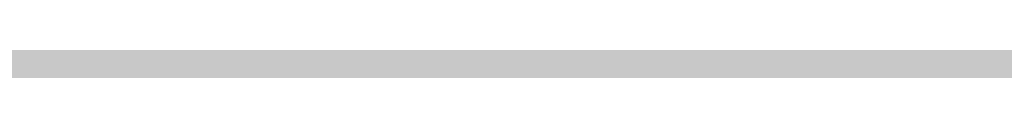
# Model space of a CAD drawing. Units: millimetres. Extents: x -22994 to 29398, y -19990 to 20176.
# Tile 90 of 135: x 229.428 to 230.597, y 83.535 to 83.549. Entities that reach past the tile are written whole.
import ezdxf
from ezdxf import colors
from ezdxf.entities.mleader import LeaderData, LeaderLine
from ezdxf.math import Vec2, Vec3

# ---------------------------------------------------------------- set-up
doc = ezdxf.new("R2010")
doc.units = ezdxf.units.MM
doc.header["$MEASUREMENT"] = 0
doc.layers.add('M-ANNO-TEXT', color=7, linetype='Continuous', lineweight=25)
doc.layers.add('M-DIMS', color=2, linetype='Continuous', lineweight=18)
doc.styles.get("Standard").update_dxf_attribs({"font": 'arial.ttf'})
doc.dimstyles.get("Standard").update_dxf_attribs({"dimtxt": 0.18, "dimasz": 10000, "dimexe": 0.18, "dimexo": 0.0625, "dimgap": 0.09, "dimtad": 0, "dimtih": 1, "dimtoh": 1, "dimdec": 0, "dimzin": 0, "dimdsep": 46, "dimtxsty": 'Standard', "dimcen": 0.09, "dimadec": 0, "dimazin": 0, "dimtfac": 1, "dimtdec": 0, "dimtofl": 0, "dimtmove": 0, "dimatfit": 3, "dimfxl": 1, "dimtolj": 1, "dimtzin": 0, "dimlwd": 30, "dimarcsym": 0})

# ---------------------------------------------------------------- blocks, each defined once
blk = doc.blocks.new('*D2')
at = {"layer": 'Defpoints', "color": 0, "transparency": 16777216}
for p in [(6.6773, 10.2713), (290.852, 10.2713), (290.852, -5.0787)]:
    blk.add_point(p, dxfattribs=at)
at = {"layer": 'M-DIMS', "color": 0, "lineweight": -2, "transparency": 16777216}
for p, q in [((6.6773, 10.2088), (6.6773, -5.2587)), ((290.852, 10.2088), (290.852, -5.2587))]:
    blk.add_line(p, q, dxfattribs=at)
at = {"layer": 'M-DIMS', "color": 0, "lineweight": 30, "transparency": 16777216}
for p, q in [((-9993.3227, -5.0787), (-19993.3227, -5.0787)), ((10290.852, -5.0787), (20290.852, -5.0787))]:
    blk.add_line(p, q, dxfattribs=at)
at = {"layer": 'M-DIMS', "color": 0, "transparency": 16777216}
for points in [[(-9993.3227, 1661.5879), (-9993.3227, -1671.7454), (6.6773, -5.0787)], [(10290.852, 1661.5879), (10290.852, -1671.7454), (290.852, -5.0787)]]:
    blk.add_solid(points, dxfattribs=at)
at = {"layer": 'M-DIMS', "color": 0, "transparency": 16777216, "insert": (148.7647, -5.0787), "char_height": 0.18, "attachment_point": 5}
blk.add_mtext('\\A1;284.2', dxfattribs=at)
blk = doc.blocks.new('*D3')
at = {"layer": 'Defpoints', "color": 0, "transparency": 16777216}
for p in [(110.2647, 204.1654), (110.2647, 176.3662), (95.8327, 127.967)]:
    blk.add_point(p, dxfattribs=at)
at = {"layer": 'M-DIMS', "color": 0, "lineweight": -2, "transparency": 16777216}
for p, q in [((95.8327, 128.0295), (95.8327, 204.3454)), ((110.2647, 176.4287), (110.2647, 204.3454))]:
    blk.add_line(p, q, dxfattribs=at)
at = {"layer": 'M-DIMS', "color": 0, "lineweight": 30, "transparency": 16777216}
for p, q in [((-9904.1673, 204.1654), (-19904.1673, 204.1654)), ((10110.2647, 204.1654), (20110.2647, 204.1654))]:
    blk.add_line(p, q, dxfattribs=at)
at = {"layer": 'M-DIMS', "color": 0, "transparency": 16777216}
for points in [[(-9904.1673, 1870.8321), (-9904.1673, -1462.5013), (95.8327, 204.1654)], [(10110.2647, 1870.8321), (10110.2647, -1462.5013), (110.2647, 204.1654)]]:
    blk.add_solid(points, dxfattribs=at)
at = {"layer": 'M-DIMS', "color": 0, "transparency": 16777216, "insert": (103.0487, 204.1654), "char_height": 0.18, "attachment_point": 5}
blk.add_mtext('\\A1;14.432', dxfattribs=at)
blk = doc.blocks.new('*D4')
at = {"layer": 'Defpoints', "color": 0, "transparency": 16777216}
for p in [(116.2647, 204.1654), (110.2647, 176.3662), (116.2647, 176.3662)]:
    blk.add_point(p, dxfattribs=at)
at = {"layer": 'M-DIMS', "color": 0, "lineweight": -2, "transparency": 16777216}
for p, q in [((110.2647, 176.4287), (110.2647, 204.3454)), ((116.2647, 176.4287), (116.2647, 204.3454))]:
    blk.add_line(p, q, dxfattribs=at)
at = {"layer": 'M-DIMS', "color": 0, "lineweight": 30, "transparency": 16777216}
for p, q in [((-9889.7353, 204.1654), (-19889.7353, 204.1654)), ((10116.2647, 204.1654), (20116.2647, 204.1654))]:
    blk.add_line(p, q, dxfattribs=at)
at = {"layer": 'M-DIMS', "color": 0, "transparency": 16777216}
for points in [[(-9889.7353, 1870.8321), (-9889.7353, -1462.5013), (110.2647, 204.1654)], [(10116.2647, 1870.8321), (10116.2647, -1462.5013), (116.2647, 204.1654)]]:
    blk.add_solid(points, dxfattribs=at)
at = {"layer": 'M-DIMS', "color": 0, "transparency": 16777216, "insert": (113.2647, 204.1654), "char_height": 0.18, "attachment_point": 5}
blk.add_mtext('\\A1;6', dxfattribs=at)
blk = doc.blocks.new('*D5')
at = {"layer": 'Defpoints', "color": 0, "transparency": 16777216}
for p in [(181.2647, 204.1654), (116.2647, 176.3662), (181.2647, 176.3662)]:
    blk.add_point(p, dxfattribs=at)
at = {"layer": 'M-DIMS', "color": 0, "lineweight": -2, "transparency": 16777216}
for p, q in [((116.2647, 176.4287), (116.2647, 204.3454)), ((181.2647, 176.4287), (181.2647, 204.3454))]:
    blk.add_line(p, q, dxfattribs=at)
at = {"layer": 'M-DIMS', "color": 0, "lineweight": 30, "transparency": 16777216}
for p, q in [((-9883.7353, 204.1654), (-19883.7353, 204.1654)), ((10181.2647, 204.1654), (20181.2647, 204.1654))]:
    blk.add_line(p, q, dxfattribs=at)
at = {"layer": 'M-DIMS', "color": 0, "transparency": 16777216}
for points in [[(-9883.7353, 1870.8321), (-9883.7353, -1462.5013), (116.2647, 204.1654)], [(10181.2647, 1870.8321), (10181.2647, -1462.5013), (181.2647, 204.1654)]]:
    blk.add_solid(points, dxfattribs=at)
at = {"layer": 'M-DIMS', "color": 0, "transparency": 16777216, "insert": (148.7647, 204.1654), "char_height": 0.18, "attachment_point": 5}
blk.add_mtext('\\A1;65', dxfattribs=at)
blk = doc.blocks.new('*D6')
at = {"layer": 'Defpoints', "color": 0, "transparency": 16777216}
for p in [(187.2647, 204.1654), (181.2647, 176.3662), (187.2647, 176.3662)]:
    blk.add_point(p, dxfattribs=at)
at = {"layer": 'M-DIMS', "color": 0, "lineweight": -2, "transparency": 16777216}
for p, q in [((181.2647, 176.4287), (181.2647, 204.3454)), ((187.2647, 176.4287), (187.2647, 204.3454))]:
    blk.add_line(p, q, dxfattribs=at)
at = {"layer": 'M-DIMS', "color": 0, "lineweight": 30, "transparency": 16777216}
for p, q in [((-9818.7353, 204.1654), (-19818.7353, 204.1654)), ((10187.2647, 204.1654), (20187.2647, 204.1654))]:
    blk.add_line(p, q, dxfattribs=at)
at = {"layer": 'M-DIMS', "color": 0, "transparency": 16777216}
for points in [[(-9818.7353, 1870.8321), (-9818.7353, -1462.5013), (181.2647, 204.1654)], [(10187.2647, 1870.8321), (10187.2647, -1462.5013), (187.2647, 204.1654)]]:
    blk.add_solid(points, dxfattribs=at)
at = {"layer": 'M-DIMS', "color": 0, "transparency": 16777216, "insert": (184.2647, 204.1654), "char_height": 0.18, "attachment_point": 5}
blk.add_mtext('\\A1;6', dxfattribs=at)
blk = doc.blocks.new('*D7')
at = {"layer": 'Defpoints', "color": 0, "transparency": 16777216}
for p in [(201.6967, 204.1654), (187.2647, 176.3662), (201.6967, 127.967)]:
    blk.add_point(p, dxfattribs=at)
at = {"layer": 'M-DIMS', "color": 0, "lineweight": -2, "transparency": 16777216}
for p, q in [((187.2647, 176.4287), (187.2647, 204.3454)), ((201.6967, 128.0295), (201.6967, 204.3454))]:
    blk.add_line(p, q, dxfattribs=at)
at = {"layer": 'M-DIMS', "color": 0, "lineweight": 30, "transparency": 16777216}
for p, q in [((-9812.7353, 204.1654), (-19812.7353, 204.1654)), ((10201.6967, 204.1654), (20201.6967, 204.1654))]:
    blk.add_line(p, q, dxfattribs=at)
at = {"layer": 'M-DIMS', "color": 0, "transparency": 16777216}
for points in [[(-9812.7353, 1870.8321), (-9812.7353, -1462.5013), (187.2647, 204.1654)], [(10201.6967, 1870.8321), (10201.6967, -1462.5013), (201.6967, 204.1654)]]:
    blk.add_solid(points, dxfattribs=at)
at = {"layer": 'M-DIMS', "color": 0, "transparency": 16777216, "insert": (194.4807, 204.1654), "char_height": 0.18, "attachment_point": 5}
blk.add_mtext('\\A1;14.432', dxfattribs=at)
blk = doc.blocks.new('*D8')
at = {"layer": 'Defpoints', "color": 0, "transparency": 16777216}
for p in [(227.6485, 204.1654), (227.6485, 146.7296), (201.6967, 127.967)]:
    blk.add_point(p, dxfattribs=at)
at = {"layer": 'M-DIMS', "color": 0, "lineweight": -2, "transparency": 16777216}
for p, q in [((201.6967, 128.0295), (201.6967, 204.3454)), ((227.6485, 146.7921), (227.6485, 204.3454))]:
    blk.add_line(p, q, dxfattribs=at)
at = {"layer": 'M-DIMS', "color": 0, "lineweight": 30, "transparency": 16777216}
for p, q in [((-9798.3033, 204.1654), (-19798.3033, 204.1654)), ((10227.6485, 204.1654), (20227.6485, 204.1654))]:
    blk.add_line(p, q, dxfattribs=at)
at = {"layer": 'M-DIMS', "color": 0, "transparency": 16777216}
for points in [[(-9798.3033, 1870.8321), (-9798.3033, -1462.5013), (201.6967, 204.1654)], [(10227.6485, 1870.8321), (10227.6485, -1462.5013), (227.6485, 204.1654)]]:
    blk.add_solid(points, dxfattribs=at)
at = {"layer": 'M-DIMS', "color": 0, "transparency": 16777216, "insert": (214.6726, 204.1654), "char_height": 0.18, "attachment_point": 5}
blk.add_mtext('\\A1;25.95', dxfattribs=at)
blk = doc.blocks.new('*D9')
at = {"layer": 'Defpoints', "color": 0, "transparency": 16777216}
for p in [(187.2647, 176.3662), (306.202, 176.3662), (290.852, 10.2713)]:
    blk.add_point(p, dxfattribs=at)
at = {"layer": 'M-DIMS', "color": 0, "lineweight": 30, "transparency": 16777216}
for p, q in [((306.202, 10176.3662), (306.202, 20176.3662)), ((306.202, -9989.7287), (306.202, -19989.7287))]:
    blk.add_line(p, q, dxfattribs=at)
at = {"layer": 'M-DIMS', "color": 0, "lineweight": -2, "transparency": 16777216}
for p, q in [((187.3272, 176.3662), (306.382, 176.3662)), ((290.9145, 10.2713), (306.382, 10.2713))]:
    blk.add_line(p, q, dxfattribs=at)
at = {"layer": 'M-DIMS', "color": 0, "transparency": 16777216}
for points in [[(-1360.4646, 10176.3662), (1972.8687, 10176.3662), (306.202, 176.3662)], [(-1360.4646, -9989.7287), (1972.8687, -9989.7287), (306.202, 10.2713)]]:
    blk.add_solid(points, dxfattribs=at)
at = {"layer": 'M-DIMS', "color": 0, "transparency": 16777216, "insert": (306.202, 93.3187), "char_height": 0.18, "attachment_point": 5}
blk.add_mtext('\\A1;166.1', dxfattribs=at)
blk = doc.blocks.new('*D10')
at = {"layer": 'Defpoints', "color": 0, "transparency": 16777216}
for p in [(125.6498, 136.0713), (133.3459, 136.0713), (133.3459, -5.0787)]:
    blk.add_point(p, dxfattribs=at)
at = {"layer": 'M-DIMS', "color": 0, "lineweight": -2, "transparency": 16777216}
for p, q in [((125.6498, 136.0088), (125.6498, -5.2587)), ((133.3459, 136.0088), (133.3459, -5.2587))]:
    blk.add_line(p, q, dxfattribs=at)
at = {"layer": 'M-DIMS', "color": 0, "lineweight": 30, "transparency": 16777216}
for p, q in [((-9874.3502, -5.0787), (-19874.3502, -5.0787)), ((10133.3459, -5.0787), (20133.3459, -5.0787))]:
    blk.add_line(p, q, dxfattribs=at)
at = {"layer": 'M-DIMS', "color": 0, "transparency": 16777216}
for points in [[(-9874.3502, 1661.5879), (-9874.3502, -1671.7454), (125.6498, -5.0787)], [(10133.3459, 1661.5879), (10133.3459, -1671.7454), (133.3459, -5.0787)]]:
    blk.add_solid(points, dxfattribs=at)
at = {"layer": 'M-DIMS', "color": 0, "transparency": 16777216, "insert": (129.4978, -5.0787), "char_height": 0.18, "attachment_point": 5}
blk.add_mtext('\\A1;7.696', dxfattribs=at)
blk = doc.blocks.new('*D11')
at = {"layer": 'Defpoints', "color": 0, "transparency": 16777216}
for p in [(133.3459, 136.0713), (135.6498, 136.0713), (135.6498, -5.0787)]:
    blk.add_point(p, dxfattribs=at)
at = {"layer": 'M-DIMS', "color": 0, "lineweight": -2, "transparency": 16777216}
for p, q in [((133.3459, 136.0088), (133.3459, -5.2587)), ((135.6498, 136.0088), (135.6498, -5.2587))]:
    blk.add_line(p, q, dxfattribs=at)
at = {"layer": 'M-DIMS', "color": 0, "lineweight": 30, "transparency": 16777216}
for p, q in [((-9866.6541, -5.0787), (-19866.6541, -5.0787)), ((10135.6498, -5.0787), (20135.6498, -5.0787))]:
    blk.add_line(p, q, dxfattribs=at)
at = {"layer": 'M-DIMS', "color": 0, "transparency": 16777216}
for points in [[(-9866.6541, 1661.5879), (-9866.6541, -1671.7454), (133.3459, -5.0787)], [(10135.6498, 1661.5879), (10135.6498, -1671.7454), (135.6498, -5.0787)]]:
    blk.add_solid(points, dxfattribs=at)
at = {"layer": 'M-DIMS', "color": 0, "transparency": 16777216, "insert": (134.4978, -5.0787), "char_height": 0.18, "attachment_point": 5}
blk.add_mtext('\\A1;2.304', dxfattribs=at)
blk = doc.blocks.new('*D12')
at = {"layer": 'Defpoints', "color": 0, "transparency": 16777216}
for p in [(135.6498, 136.0713), (145.6498, 136.0713), (145.6498, -5.0787)]:
    blk.add_point(p, dxfattribs=at)
at = {"layer": 'M-DIMS', "color": 0, "lineweight": -2, "transparency": 16777216}
for p, q in [((135.6498, 136.0088), (135.6498, -5.2587)), ((145.6498, 136.0088), (145.6498, -5.2587))]:
    blk.add_line(p, q, dxfattribs=at)
at = {"layer": 'M-DIMS', "color": 0, "lineweight": 30, "transparency": 16777216}
for p, q in [((-9864.3502, -5.0787), (-19864.3502, -5.0787)), ((10145.6498, -5.0787), (20145.6498, -5.0787))]:
    blk.add_line(p, q, dxfattribs=at)
at = {"layer": 'M-DIMS', "color": 0, "transparency": 16777216}
for points in [[(-9864.3502, 1661.5879), (-9864.3502, -1671.7454), (135.6498, -5.0787)], [(10145.6498, 1661.5879), (10145.6498, -1671.7454), (145.6498, -5.0787)]]:
    blk.add_solid(points, dxfattribs=at)
at = {"layer": 'M-DIMS', "color": 0, "transparency": 16777216, "insert": (140.6498, -5.0787), "char_height": 0.18, "attachment_point": 5}
blk.add_mtext('\\A1;10', dxfattribs=at)
blk = doc.blocks.new('*D13')
at = {"layer": 'Defpoints', "color": 0, "transparency": 16777216}
for p in [(145.6498, 136.0713), (155.6498, 136.0713), (155.6498, -5.0787)]:
    blk.add_point(p, dxfattribs=at)
at = {"layer": 'M-DIMS', "color": 0, "lineweight": -2, "transparency": 16777216}
for p, q in [((145.6498, 136.0088), (145.6498, -5.2587)), ((155.6498, 136.0088), (155.6498, -5.2587))]:
    blk.add_line(p, q, dxfattribs=at)
at = {"layer": 'M-DIMS', "color": 0, "lineweight": 30, "transparency": 16777216}
for p, q in [((-9854.3502, -5.0787), (-19854.3502, -5.0787)), ((10155.6498, -5.0787), (20155.6498, -5.0787))]:
    blk.add_line(p, q, dxfattribs=at)
at = {"layer": 'M-DIMS', "color": 0, "transparency": 16777216}
for points in [[(-9854.3502, 1661.5879), (-9854.3502, -1671.7454), (145.6498, -5.0787)], [(10155.6498, 1661.5879), (10155.6498, -1671.7454), (155.6498, -5.0787)]]:
    blk.add_solid(points, dxfattribs=at)
at = {"layer": 'M-DIMS', "color": 0, "transparency": 16777216, "insert": (150.6498, -5.0787), "char_height": 0.18, "attachment_point": 5}
blk.add_mtext('\\A1;10', dxfattribs=at)
blk = doc.blocks.new('*D14')
at = {"layer": 'Defpoints', "color": 0, "transparency": 16777216}
for p in [(155.6498, 136.0713), (165.6498, 136.0713), (165.6498, -5.0787)]:
    blk.add_point(p, dxfattribs=at)
at = {"layer": 'M-DIMS', "color": 0, "lineweight": -2, "transparency": 16777216}
for p, q in [((155.6498, 136.0088), (155.6498, -5.2587)), ((165.6498, 136.0088), (165.6498, -5.2587))]:
    blk.add_line(p, q, dxfattribs=at)
at = {"layer": 'M-DIMS', "color": 0, "lineweight": 30, "transparency": 16777216}
for p, q in [((-9844.3502, -5.0787), (-19844.3502, -5.0787)), ((10165.6498, -5.0787), (20165.6498, -5.0787))]:
    blk.add_line(p, q, dxfattribs=at)
at = {"layer": 'M-DIMS', "color": 0, "transparency": 16777216}
for points in [[(-9844.3502, 1661.5879), (-9844.3502, -1671.7454), (155.6498, -5.0787)], [(10165.6498, 1661.5879), (10165.6498, -1671.7454), (165.6498, -5.0787)]]:
    blk.add_solid(points, dxfattribs=at)
at = {"layer": 'M-DIMS', "color": 0, "transparency": 16777216, "insert": (160.6498, -5.0787), "char_height": 0.18, "attachment_point": 5}
blk.add_mtext('\\A1;10', dxfattribs=at)
blk = doc.blocks.new('*D15')
at = {"layer": 'Defpoints', "color": 0, "transparency": 16777216}
for p in [(173.3459, 154.788), (173.3459, 136.0713), (306.202, 136.0713)]:
    blk.add_point(p, dxfattribs=at)
at = {"layer": 'M-DIMS', "color": 0, "lineweight": 30, "transparency": 16777216}
for p, q in [((306.202, 10154.788), (306.202, 20154.788)), ((306.202, -9863.9287), (306.202, -19863.9287))]:
    blk.add_line(p, q, dxfattribs=at)
at = {"layer": 'M-DIMS', "color": 0, "lineweight": -2, "transparency": 16777216}
for p, q in [((173.4084, 154.788), (306.382, 154.788)), ((173.4084, 136.0713), (306.382, 136.0713))]:
    blk.add_line(p, q, dxfattribs=at)
at = {"layer": 'M-DIMS', "color": 0, "transparency": 16777216}
for points in [[(-1360.4646, 10154.788), (1972.8687, 10154.788), (306.202, 154.788)], [(-1360.4646, -9863.9287), (1972.8687, -9863.9287), (306.202, 136.0713)]]:
    blk.add_solid(points, dxfattribs=at)
at = {"layer": 'M-DIMS', "color": 0, "transparency": 16777216, "insert": (306.202, 145.4297), "char_height": 0.18, "attachment_point": 5}
blk.add_mtext('\\A1;18.717', dxfattribs=at)
blk = doc.blocks.new('*D16')
at = {"layer": 'Defpoints', "color": 0, "transparency": 16777216}
for p in [(120.1702, 204.1654), (110.4658, 48.0349), (120.1702, 48.0349)]:
    blk.add_point(p, dxfattribs=at)
at = {"layer": 'M-DIMS', "color": 0, "lineweight": -2, "transparency": 16777216}
for p, q in [((110.4658, 48.0974), (110.4658, 204.3454)), ((120.1702, 48.0974), (120.1702, 204.3454))]:
    blk.add_line(p, q, dxfattribs=at)
at = {"layer": 'M-DIMS', "color": 0, "lineweight": 30, "transparency": 16777216}
for p, q in [((-9889.5342, 204.1654), (-19889.5342, 204.1654)), ((10120.1702, 204.1654), (20120.1702, 204.1654))]:
    blk.add_line(p, q, dxfattribs=at)
at = {"layer": 'M-DIMS', "color": 0, "transparency": 16777216}
for points in [[(-9889.5342, 1870.8321), (-9889.5342, -1462.5013), (110.4658, 204.1654)], [(10120.1702, 1870.8321), (10120.1702, -1462.5013), (120.1702, 204.1654)]]:
    blk.add_solid(points, dxfattribs=at)
at = {"layer": 'M-DIMS', "color": 0, "transparency": 16777216, "insert": (115.318, 204.1654), "char_height": 0.18, "attachment_point": 5}
blk.add_mtext('\\A1;9.704', dxfattribs=at)
blk = doc.blocks.new('*D17')
at = {"layer": 'Defpoints', "color": 0, "transparency": 16777216}
for p in [(126.1702, 204.1654), (120.1702, 48.0349), (126.1702, 48.0349)]:
    blk.add_point(p, dxfattribs=at)
at = {"layer": 'M-DIMS', "color": 0, "lineweight": -2, "transparency": 16777216}
for p, q in [((120.1702, 48.0974), (120.1702, 204.3454)), ((126.1702, 48.0974), (126.1702, 204.3454))]:
    blk.add_line(p, q, dxfattribs=at)
at = {"layer": 'M-DIMS', "color": 0, "lineweight": 30, "transparency": 16777216}
for p, q in [((-9879.8298, 204.1654), (-19879.8298, 204.1654)), ((10126.1702, 204.1654), (20126.1702, 204.1654))]:
    blk.add_line(p, q, dxfattribs=at)
at = {"layer": 'M-DIMS', "color": 0, "transparency": 16777216}
for points in [[(-9879.8298, 1870.8321), (-9879.8298, -1462.5013), (120.1702, 204.1654)], [(10126.1702, 1870.8321), (10126.1702, -1462.5013), (126.1702, 204.1654)]]:
    blk.add_solid(points, dxfattribs=at)
at = {"layer": 'M-DIMS', "color": 0, "transparency": 16777216, "insert": (123.1702, 204.1654), "char_height": 0.18, "attachment_point": 5}
blk.add_mtext('\\A1;6', dxfattribs=at)
blk = doc.blocks.new('*D18')
at = {"layer": 'Defpoints', "color": 0, "transparency": 16777216}
for p in [(132.1702, 204.1654), (126.1702, 48.0349), (132.1702, 48.0349)]:
    blk.add_point(p, dxfattribs=at)
at = {"layer": 'M-DIMS', "color": 0, "lineweight": -2, "transparency": 16777216}
for p, q in [((126.1702, 48.0974), (126.1702, 204.3454)), ((132.1702, 48.0974), (132.1702, 204.3454))]:
    blk.add_line(p, q, dxfattribs=at)
at = {"layer": 'M-DIMS', "color": 0, "lineweight": 30, "transparency": 16777216}
for p, q in [((-9873.8298, 204.1654), (-19873.8298, 204.1654)), ((10132.1702, 204.1654), (20132.1702, 204.1654))]:
    blk.add_line(p, q, dxfattribs=at)
at = {"layer": 'M-DIMS', "color": 0, "transparency": 16777216}
for points in [[(-9873.8298, 1870.8321), (-9873.8298, -1462.5013), (126.1702, 204.1654)], [(10132.1702, 1870.8321), (10132.1702, -1462.5013), (132.1702, 204.1654)]]:
    blk.add_solid(points, dxfattribs=at)
at = {"layer": 'M-DIMS', "color": 0, "transparency": 16777216, "insert": (129.1702, 204.1654), "char_height": 0.18, "attachment_point": 5}
blk.add_mtext('\\A1;6', dxfattribs=at)
blk = doc.blocks.new('*D19')
at = {"layer": 'Defpoints', "color": 0, "transparency": 16777216}
for p in [(138.1702, 204.1654), (132.1702, 48.0349), (138.1702, 48.0349)]:
    blk.add_point(p, dxfattribs=at)
at = {"layer": 'M-DIMS', "color": 0, "lineweight": -2, "transparency": 16777216}
for p, q in [((132.1702, 48.0974), (132.1702, 204.3454)), ((138.1702, 48.0974), (138.1702, 204.3454))]:
    blk.add_line(p, q, dxfattribs=at)
at = {"layer": 'M-DIMS', "color": 0, "lineweight": 30, "transparency": 16777216}
for p, q in [((-9867.8298, 204.1654), (-19867.8298, 204.1654)), ((10138.1702, 204.1654), (20138.1702, 204.1654))]:
    blk.add_line(p, q, dxfattribs=at)
at = {"layer": 'M-DIMS', "color": 0, "transparency": 16777216}
for points in [[(-9867.8298, 1870.8321), (-9867.8298, -1462.5013), (132.1702, 204.1654)], [(10138.1702, 1870.8321), (10138.1702, -1462.5013), (138.1702, 204.1654)]]:
    blk.add_solid(points, dxfattribs=at)
at = {"layer": 'M-DIMS', "color": 0, "transparency": 16777216, "insert": (135.1702, 204.1654), "char_height": 0.18, "attachment_point": 5}
blk.add_mtext('\\A1;6', dxfattribs=at)
blk = doc.blocks.new('*D20')
at = {"layer": 'Defpoints', "color": 0, "transparency": 16777216}
for p in [(144.1702, 204.1654), (138.1702, 48.0349), (144.1702, 48.0349)]:
    blk.add_point(p, dxfattribs=at)
at = {"layer": 'M-DIMS', "color": 0, "lineweight": -2, "transparency": 16777216}
for p, q in [((138.1702, 48.0974), (138.1702, 204.3454)), ((144.1702, 48.0974), (144.1702, 204.3454))]:
    blk.add_line(p, q, dxfattribs=at)
at = {"layer": 'M-DIMS', "color": 0, "lineweight": 30, "transparency": 16777216}
for p, q in [((-9861.8298, 204.1654), (-19861.8298, 204.1654)), ((10144.1702, 204.1654), (20144.1702, 204.1654))]:
    blk.add_line(p, q, dxfattribs=at)
at = {"layer": 'M-DIMS', "color": 0, "transparency": 16777216}
for points in [[(-9861.8298, 1870.8321), (-9861.8298, -1462.5013), (138.1702, 204.1654)], [(10144.1702, 1870.8321), (10144.1702, -1462.5013), (144.1702, 204.1654)]]:
    blk.add_solid(points, dxfattribs=at)
at = {"layer": 'M-DIMS', "color": 0, "transparency": 16777216, "insert": (141.1702, 204.1654), "char_height": 0.18, "attachment_point": 5}
blk.add_mtext('\\A1;6', dxfattribs=at)
blk = doc.blocks.new('*D21')
at = {"layer": 'Defpoints', "color": 0, "transparency": 16777216}
for p in [(149.1157, 204.1654), (144.1702, 48.0349), (149.1157, 48.0349)]:
    blk.add_point(p, dxfattribs=at)
at = {"layer": 'M-DIMS', "color": 0, "lineweight": -2, "transparency": 16777216}
for p, q in [((144.1702, 48.0974), (144.1702, 204.3454)), ((149.1157, 48.0974), (149.1157, 204.3454))]:
    blk.add_line(p, q, dxfattribs=at)
at = {"layer": 'M-DIMS', "color": 0, "lineweight": 30, "transparency": 16777216}
for p, q in [((-9855.8298, 204.1654), (-19855.8298, 204.1654)), ((10149.1157, 204.1654), (20149.1157, 204.1654))]:
    blk.add_line(p, q, dxfattribs=at)
at = {"layer": 'M-DIMS', "color": 0, "transparency": 16777216}
for points in [[(-9855.8298, 1870.8321), (-9855.8298, -1462.5013), (144.1702, 204.1654)], [(10149.1157, 1870.8321), (10149.1157, -1462.5013), (149.1157, 204.1654)]]:
    blk.add_solid(points, dxfattribs=at)
at = {"layer": 'M-DIMS', "color": 0, "transparency": 16777216, "insert": (146.6429, 204.1654), "char_height": 0.18, "attachment_point": 5}
blk.add_mtext('\\A1;4.945', dxfattribs=at)
blk = doc.blocks.new('*D22')
at = {"layer": 'Defpoints', "color": 0, "transparency": 16777216}
for p in [(149.1157, 30.9895), (155.1157, 30.9895), (155.1157, -5.0787)]:
    blk.add_point(p, dxfattribs=at)
at = {"layer": 'M-DIMS', "color": 0, "lineweight": -2, "transparency": 16777216}
for p, q in [((149.1157, 30.927), (149.1157, -5.2587)), ((155.1157, 30.927), (155.1157, -5.2587))]:
    blk.add_line(p, q, dxfattribs=at)
at = {"layer": 'M-DIMS', "color": 0, "lineweight": 30, "transparency": 16777216}
for p, q in [((-9850.8843, -5.0787), (-19850.8843, -5.0787)), ((10155.1157, -5.0787), (20155.1157, -5.0787))]:
    blk.add_line(p, q, dxfattribs=at)
at = {"layer": 'M-DIMS', "color": 0, "transparency": 16777216}
for points in [[(-9850.8843, 1661.5879), (-9850.8843, -1671.7454), (149.1157, -5.0787)], [(10155.1157, 1661.5879), (10155.1157, -1671.7454), (155.1157, -5.0787)]]:
    blk.add_solid(points, dxfattribs=at)
at = {"layer": 'M-DIMS', "color": 0, "transparency": 16777216, "insert": (152.1157, -5.0787), "char_height": 0.18, "attachment_point": 5}
blk.add_mtext('\\A1;6', dxfattribs=at)
blk = doc.blocks.new('*D23')
at = {"layer": 'Defpoints', "color": 0, "transparency": 16777216}
for p in [(155.1157, 30.9895), (161.1157, 30.9895), (161.1157, -5.0787)]:
    blk.add_point(p, dxfattribs=at)
at = {"layer": 'M-DIMS', "color": 0, "lineweight": -2, "transparency": 16777216}
for p, q in [((155.1157, 30.927), (155.1157, -5.2587)), ((161.1157, 30.927), (161.1157, -5.2587))]:
    blk.add_line(p, q, dxfattribs=at)
at = {"layer": 'M-DIMS', "color": 0, "lineweight": 30, "transparency": 16777216}
for p, q in [((-9844.8843, -5.0787), (-19844.8843, -5.0787)), ((10161.1157, -5.0787), (20161.1157, -5.0787))]:
    blk.add_line(p, q, dxfattribs=at)
at = {"layer": 'M-DIMS', "color": 0, "transparency": 16777216}
for points in [[(-9844.8843, 1661.5879), (-9844.8843, -1671.7454), (155.1157, -5.0787)], [(10161.1157, 1661.5879), (10161.1157, -1671.7454), (161.1157, -5.0787)]]:
    blk.add_solid(points, dxfattribs=at)
at = {"layer": 'M-DIMS', "color": 0, "transparency": 16777216, "insert": (158.1157, -5.0787), "char_height": 0.18, "attachment_point": 5}
blk.add_mtext('\\A1;6', dxfattribs=at)
blk = doc.blocks.new('*D24')
at = {"layer": 'Defpoints', "color": 0, "transparency": 16777216}
for p in [(161.1157, 30.9895), (166.4387, 30.9895), (166.4387, -5.0787)]:
    blk.add_point(p, dxfattribs=at)
at = {"layer": 'M-DIMS', "color": 0, "lineweight": -2, "transparency": 16777216}
for p, q in [((161.1157, 30.927), (161.1157, -5.2587)), ((166.4387, 30.927), (166.4387, -5.2587))]:
    blk.add_line(p, q, dxfattribs=at)
at = {"layer": 'M-DIMS', "color": 0, "lineweight": 30, "transparency": 16777216}
for p, q in [((-9838.8843, -5.0787), (-19838.8843, -5.0787)), ((10166.4387, -5.0787), (20166.4387, -5.0787))]:
    blk.add_line(p, q, dxfattribs=at)
at = {"layer": 'M-DIMS', "color": 0, "transparency": 16777216}
for points in [[(-9838.8843, 1661.5879), (-9838.8843, -1671.7454), (161.1157, -5.0787)], [(10166.4387, 1661.5879), (10166.4387, -1671.7454), (166.4387, -5.0787)]]:
    blk.add_solid(points, dxfattribs=at)
at = {"layer": 'M-DIMS', "color": 0, "transparency": 16777216, "insert": (163.7772, -5.0787), "char_height": 0.18, "attachment_point": 5}
blk.add_mtext('\\A1;5.323', dxfattribs=at)
blk = doc.blocks.new('*D25')
at = {"layer": 'Defpoints', "color": 0, "transparency": 16777216}
for p in [(166.4387, 30.9895), (172.4387, 30.9895), (172.4387, -5.0787)]:
    blk.add_point(p, dxfattribs=at)
at = {"layer": 'M-DIMS', "color": 0, "lineweight": -2, "transparency": 16777216}
for p, q in [((166.4387, 30.927), (166.4387, -5.2587)), ((172.4387, 30.927), (172.4387, -5.2587))]:
    blk.add_line(p, q, dxfattribs=at)
at = {"layer": 'M-DIMS', "color": 0, "lineweight": 30, "transparency": 16777216}
for p, q in [((-9833.5613, -5.0787), (-19833.5613, -5.0787)), ((10172.4387, -5.0787), (20172.4387, -5.0787))]:
    blk.add_line(p, q, dxfattribs=at)
at = {"layer": 'M-DIMS', "color": 0, "transparency": 16777216}
for points in [[(-9833.5613, 1661.5879), (-9833.5613, -1671.7454), (166.4387, -5.0787)], [(10172.4387, 1661.5879), (10172.4387, -1671.7454), (172.4387, -5.0787)]]:
    blk.add_solid(points, dxfattribs=at)
at = {"layer": 'M-DIMS', "color": 0, "transparency": 16777216, "insert": (169.4387, -5.0787), "char_height": 0.18, "attachment_point": 5}
blk.add_mtext('\\A1;6', dxfattribs=at)
blk = doc.blocks.new('*D26')
at = {"layer": 'Defpoints', "color": 0, "transparency": 16777216}
for p in [(172.4387, 30.9895), (178.4387, 30.9895), (178.4387, -5.0787)]:
    blk.add_point(p, dxfattribs=at)
at = {"layer": 'M-DIMS', "color": 0, "lineweight": -2, "transparency": 16777216}
for p, q in [((172.4387, 30.927), (172.4387, -5.2587)), ((178.4387, 30.927), (178.4387, -5.2587))]:
    blk.add_line(p, q, dxfattribs=at)
at = {"layer": 'M-DIMS', "color": 0, "lineweight": 30, "transparency": 16777216}
for p, q in [((-9827.5613, -5.0787), (-19827.5613, -5.0787)), ((10178.4387, -5.0787), (20178.4387, -5.0787))]:
    blk.add_line(p, q, dxfattribs=at)
at = {"layer": 'M-DIMS', "color": 0, "transparency": 16777216}
for points in [[(-9827.5613, 1661.5879), (-9827.5613, -1671.7454), (172.4387, -5.0787)], [(10178.4387, 1661.5879), (10178.4387, -1671.7454), (178.4387, -5.0787)]]:
    blk.add_solid(points, dxfattribs=at)
at = {"layer": 'M-DIMS', "color": 0, "transparency": 16777216, "insert": (175.4387, -5.0787), "char_height": 0.18, "attachment_point": 5}
blk.add_mtext('\\A1;6', dxfattribs=at)
blk = doc.blocks.new('*D27')
at = {"layer": 'Defpoints', "color": 0, "transparency": 16777216}
for p in [(178.4387, 30.9895), (188.1175, 30.9895), (188.1175, -5.0787)]:
    blk.add_point(p, dxfattribs=at)
at = {"layer": 'M-DIMS', "color": 0, "lineweight": -2, "transparency": 16777216}
for p, q in [((178.4387, 30.927), (178.4387, -5.2587)), ((188.1175, 30.927), (188.1175, -5.2587))]:
    blk.add_line(p, q, dxfattribs=at)
at = {"layer": 'M-DIMS', "color": 0, "lineweight": 30, "transparency": 16777216}
for p, q in [((-9821.5613, -5.0787), (-19821.5613, -5.0787)), ((10188.1175, -5.0787), (20188.1175, -5.0787))]:
    blk.add_line(p, q, dxfattribs=at)
at = {"layer": 'M-DIMS', "color": 0, "transparency": 16777216}
for points in [[(-9821.5613, 1661.5879), (-9821.5613, -1671.7454), (178.4387, -5.0787)], [(10188.1175, 1661.5879), (10188.1175, -1671.7454), (188.1175, -5.0787)]]:
    blk.add_solid(points, dxfattribs=at)
at = {"layer": 'M-DIMS', "color": 0, "transparency": 16777216, "insert": (183.2781, -5.0787), "char_height": 0.18, "attachment_point": 5}
blk.add_mtext('\\A1;9.679', dxfattribs=at)
blk = doc.blocks.new('*D28')
at = {"layer": 'Defpoints', "color": 0, "transparency": 16777216}
for p in [(188.1175, 48.0349), (306.202, 48.0349), (188.1175, 30.9895)]:
    blk.add_point(p, dxfattribs=at)
at = {"layer": 'M-DIMS', "color": 0, "lineweight": 30, "transparency": 16777216}
for p, q in [((306.202, 10048.0349), (306.202, 20048.0349)), ((306.202, -9969.0105), (306.202, -19969.0105))]:
    blk.add_line(p, q, dxfattribs=at)
at = {"layer": 'M-DIMS', "color": 0, "lineweight": -2, "transparency": 16777216}
for p, q in [((188.18, 48.0349), (306.382, 48.0349)), ((188.18, 30.9895), (306.382, 30.9895))]:
    blk.add_line(p, q, dxfattribs=at)
at = {"layer": 'M-DIMS', "color": 0, "transparency": 16777216}
for points in [[(-1360.4646, 10048.0349), (1972.8687, 10048.0349), (306.202, 48.0349)], [(-1360.4646, -9969.0105), (1972.8687, -9969.0105), (306.202, 30.9895)]]:
    blk.add_solid(points, dxfattribs=at)
at = {"layer": 'M-DIMS', "color": 0, "transparency": 16777216, "insert": (306.202, 39.5122), "char_height": 0.18, "attachment_point": 5}
blk.add_mtext('\\A1;17.045', dxfattribs=at)
blk = doc.blocks.new('*D29')
at = {"layer": 'Defpoints', "color": 0, "transparency": 16777216}
for p in [(36.8006, 80.045), (64.0296, 80.045)]:
    blk.add_point(p, dxfattribs=at)
at = {"layer": 'M-DIMS', "color": 0, "lineweight": -2, "transparency": 16777216}
for p, q in [((50.4151, 79.955), (50.4151, 80.135)), ((50.3251, 80.045), (50.5051, 80.045))]:
    blk.add_line(p, q, dxfattribs=at)
at = {"layer": 'M-DIMS', "color": 0, "lineweight": 30, "transparency": 16777216}
blk.add_line((20064.0296, 80.0303), (10064.0296, 80.0377), dxfattribs=at)
at = {"layer": 'M-DIMS', "color": 0, "transparency": 16777216}
blk.add_solid([(10064.0309, 1746.7043), (10064.0284, -1586.629), (64.0296, 80.045)], dxfattribs=at)
at = {"layer": 'M-DIMS', "color": 0, "transparency": 16777216, "insert": (20064.5213, 80.0303), "char_height": 0.18, "attachment_point": 5}
blk.add_mtext('\\A1;∅27.23', dxfattribs=at)
blk = doc.blocks.new('*D30')
at = {"layer": 'Defpoints', "color": 0, "transparency": 16777216}
for p in [(216.3148, 146.7291), (238.9821, 146.73)]:
    blk.add_point(p, dxfattribs=at)
at = {"layer": 'M-DIMS', "color": 0, "lineweight": 30, "transparency": 16777216}
blk.add_line((20238.9821, 147.4959), (10238.9821, 147.1129), dxfattribs=at)
at = {"layer": 'M-DIMS', "color": 0, "lineweight": -2, "transparency": 16777216}
for p, q in [((227.6485, 146.6396), (227.6485, 146.8196)), ((227.5585, 146.7296), (227.7385, 146.7296))]:
    blk.add_line(p, q, dxfattribs=at)
at = {"layer": 'M-DIMS', "color": 0, "transparency": 16777216}
blk.add_solid([(10238.9183, 1813.7796), (10239.0459, -1519.5537), (238.9821, 146.73)], dxfattribs=at)
at = {"layer": 'M-DIMS', "color": 0, "transparency": 16777216, "insert": (20239.5436, 147.4959), "char_height": 0.18, "attachment_point": 5}
blk.add_mtext('\\A1;∅22.667', dxfattribs=at)
blk = doc.blocks.new('*D31')
at = {"layer": 'Defpoints', "color": 0, "transparency": 16777216}
for p in [(223.1641, 146.7291), (232.1328, 146.73)]:
    blk.add_point(p, dxfattribs=at)
at = {"layer": 'M-DIMS', "color": 0, "lineweight": 30, "transparency": 16777216}
blk.add_line((20232.1327, 148.6656), (10232.1328, 147.6978), dxfattribs=at)
at = {"layer": 'M-DIMS', "color": 0, "lineweight": -2, "transparency": 16777216}
for p, q in [((227.6485, 146.6396), (227.6485, 146.8196)), ((227.5585, 146.7296), (227.7385, 146.7296))]:
    blk.add_line(p, q, dxfattribs=at)
at = {"layer": 'M-DIMS', "color": 0, "transparency": 16777216}
blk.add_solid([(10231.9715, 1814.3645), (10232.2941, -1518.9688), (232.1328, 146.73)], dxfattribs=at)
at = {"layer": 'M-DIMS', "color": 0, "transparency": 16777216, "insert": (20232.6245, 148.6656), "char_height": 0.18, "attachment_point": 5}
blk.add_mtext('\\A1;∅8.969', dxfattribs=at)
blk = doc.blocks.new('*D33')
at = {"layer": 'Defpoints', "color": 0, "transparency": 16777216}
for p in [(229.5613, 154.3773), (232.9972, 153.3509)]:
    blk.add_point(p, dxfattribs=at)
at = {"layer": 'M-DIMS', "color": 0, "lineweight": -2, "transparency": 16777216}
for p, q in [((229.5613, 154.2873), (229.5613, 154.4673)), ((229.4713, 154.3773), (229.6513, 154.3773))]:
    blk.add_line(p, q, dxfattribs=at)
at = {"layer": 'M-DIMS', "color": 0, "lineweight": 30, "transparency": 16777216}
for p, q in [((19396.3388, -5570.8378), (9814.668, -2708.7434)), ((29396.3388, -5570.8378), (19396.3388, -5570.8378))]:
    blk.add_line(p, q, dxfattribs=at)
at = {"layer": 'M-DIMS', "color": 0, "transparency": 16777216}
blk.add_solid([(10291.6837, -1111.7983), (9337.6523, -4305.6886), (232.9972, 153.3509)], dxfattribs=at)
at = {"layer": 'M-DIMS', "color": 0, "transparency": 16777216, "insert": (29397.0125, -5570.8378), "char_height": 0.18, "attachment_point": 5}
blk.add_mtext('\\A1;6X R3.586', dxfattribs=at)
blk = doc.blocks.new('*D36')
at = {"layer": 'Defpoints', "color": 0, "transparency": 16777216}
for p in [(46.39, 31.3035), (46.3875, 26.5934)]:
    blk.add_point(p, dxfattribs=at)
at = {"layer": 'M-DIMS', "color": 0, "lineweight": 30, "transparency": 16777216}
for p, q in [((57.1499, 20031.3006), (51.77, 10031.302)), ((10057.1499, 20031.3006), (57.1499, 20031.3006))]:
    blk.add_line(p, q, dxfattribs=at)
at = {"layer": 'M-DIMS', "color": 0, "lineweight": -2, "transparency": 16777216}
for p, q in [((46.3887, 28.8585), (46.3887, 29.0385)), ((46.2987, 28.9485), (46.4787, 28.9485))]:
    blk.add_line(p, q, dxfattribs=at)
at = {"layer": 'M-DIMS', "color": 0, "transparency": 16777216}
blk.add_solid([(-1614.8965, 10032.1987), (1718.4364, 10030.4054), (46.39, 31.3035)], dxfattribs=at)
at = {"layer": 'M-DIMS', "color": 0, "transparency": 16777216, "insert": (10057.5542, 20031.3006), "char_height": 0.18, "attachment_point": 5}
blk.add_mtext('\\A1;∅4.71', dxfattribs=at)
blk = doc.blocks.new('*D37')
at = {"layer": 'Defpoints', "color": 0, "transparency": 16777216}
for p in [(54.8343, 118.6145), (59.4936, 118.614)]:
    blk.add_point(p, dxfattribs=at)
at = {"layer": 'M-DIMS', "color": 0, "lineweight": -2, "transparency": 16777216}
for p, q in [((57.1639, 118.5243), (57.1639, 118.7043)), ((57.0739, 118.6143), (57.2539, 118.6143))]:
    blk.add_line(p, q, dxfattribs=at)
at = {"layer": 'M-DIMS', "color": 0, "lineweight": 30, "transparency": 16777216}
blk.add_line((20059.4934, 116.2531), (10059.4935, 117.4336), dxfattribs=at)
at = {"layer": 'M-DIMS', "color": 0, "transparency": 16777216}
blk.add_solid([(10059.6902, 1784.1002), (10059.2968, -1549.2331), (59.4936, 118.614)], dxfattribs=at)
at = {"layer": 'M-DIMS', "color": 0, "transparency": 16777216, "insert": (20059.9852, 116.2531), "char_height": 0.18, "attachment_point": 5}
blk.add_mtext('\\A1;∅4.659', dxfattribs=at)

msp = doc.modelspace()

# ---------------------------------------------------------------- dimensions: what is measured, and where the dimension line sits
at = {"layer": 'M-DIMS'}
for base, p1, p2, override, picture, middle in [((306.202, 176.3662), (290.852, 10.2713), (187.2647, 176.3662), {"dimdec": 1, "dimlfac": 1, "dimrnd": 0, "dimzin": 0, "dimdsep": 46, "dimlunit": 2}, '*D9', (306.202, 93.3187)), ((306.202, 136.0713), (173.3459, 154.788), (173.3459, 136.0713), {"dimdec": 3, "dimlfac": 1, "dimrnd": 0, "dimzin": 0, "dimdsep": 46, "dimlunit": 2}, '*D15', (306.202, 145.4297)), ((306.202, 48.0349), (188.1175, 30.9895), (188.1175, 48.0349), {"dimdec": 3, "dimlfac": 1, "dimrnd": 0, "dimzin": 0, "dimdsep": 46, "dimlunit": 2}, '*D28', (306.202, 39.5122))]:
    dim = msp.add_linear_dim(base=base, p1=p1, p2=p2, angle=90, dimstyle='Standard', override=override, dxfattribs=at)
    dim.commit()
    dim.dimension.update_dxf_attribs({"geometry": picture, "text_midpoint": middle})
for p1, p2, override, picture, middle in [((46.3875, 26.5934), (46.39, 31.3035), {"dimdec": 2, "dimlfac": 1, "dimrnd": 0, "dimzin": 0, "dimdsep": 46, "dimlunit": 2}, '*D36', (10057.5542, 20031.3006)), ((223.1641, 146.7291), (232.1328, 146.73), {"dimdec": 3, "dimlfac": 1, "dimrnd": 0, "dimzin": 0, "dimdsep": 46, "dimlunit": 2}, '*D31', (20232.1327, 148.6656)), ((216.3148, 146.7291), (238.9821, 146.73), {"dimdec": 3, "dimlfac": 1, "dimrnd": 0, "dimzin": 0, "dimdsep": 46, "dimlunit": 2}, '*D30', (20238.9821, 147.4959))]:
    dim = msp.add_diameter_dim_2p(p1=p1, p2=p2, dimstyle='Standard', override=override, dxfattribs=at)
    dim.commit()
    dim.dimension.update_dxf_attribs({"geometry": picture, "text_midpoint": middle, "dimtype": 163})
for base, p1, p2, override, picture, middle in [((110.2647, 204.1654), (95.8327, 127.967), (110.2647, 176.3662), {"dimdec": 3, "dimlfac": 1, "dimrnd": 0, "dimzin": 0, "dimdsep": 46, "dimlunit": 2}, '*D3', (103.0487, 204.1654)), ((116.2647, 204.1654), (110.2647, 176.3662), (116.2647, 176.3662), {"dimdec": 0, "dimlfac": 1, "dimrnd": 0, "dimzin": 0, "dimdsep": 46, "dimlunit": 2}, '*D4', (113.2647, 204.1654)), ((120.1702, 204.1654), (110.4658, 48.0349), (120.1702, 48.0349), {"dimdec": 3, "dimlfac": 1, "dimrnd": 0, "dimzin": 0, "dimdsep": 46, "dimlunit": 2}, '*D16', (115.318, 204.1654)), ((181.2647, 204.1654), (116.2647, 176.3662), (181.2647, 176.3662), {"dimdec": 0, "dimlfac": 1, "dimrnd": 0, "dimzin": 0, "dimdsep": 46, "dimlunit": 2}, '*D5', (148.7647, 204.1654)), ((126.1702, 204.1654), (120.1702, 48.0349), (126.1702, 48.0349), {"dimdec": 0, "dimlfac": 1, "dimrnd": 0, "dimzin": 0, "dimdsep": 46, "dimlunit": 2}, '*D17', (123.1702, 204.1654)), ((132.1702, 204.1654), (126.1702, 48.0349), (132.1702, 48.0349), {"dimdec": 0, "dimlfac": 1, "dimrnd": 0, "dimzin": 0, "dimdsep": 46, "dimlunit": 2}, '*D18', (129.1702, 204.1654)), ((138.1702, 204.1654), (132.1702, 48.0349), (138.1702, 48.0349), {"dimdec": 0, "dimlfac": 1, "dimrnd": 0, "dimzin": 0, "dimdsep": 46, "dimlunit": 2}, '*D19', (135.1702, 204.1654)), ((144.1702, 204.1654), (138.1702, 48.0349), (144.1702, 48.0349), {"dimdec": 0, "dimlfac": 1, "dimrnd": 0, "dimzin": 0, "dimdsep": 46, "dimlunit": 2}, '*D20', (141.1702, 204.1654)), ((149.11567, 204.16539), (144.17023, 48.03494), (149.11567, 48.03494), {"dimdec": 3, "dimlfac": 1, "dimrnd": 0, "dimzin": 0, "dimdsep": 46, "dimlunit": 2}, '*D21', (146.64295, 204.16539)), ((187.2647, 204.1654), (181.2647, 176.3662), (187.2647, 176.3662), {"dimdec": 0, "dimlfac": 1, "dimrnd": 0, "dimzin": 0, "dimdsep": 46, "dimlunit": 2}, '*D6', (184.2647, 204.1654)), ((201.6967, 204.1654), (187.2647, 176.3662), (201.6967, 127.967), {"dimdec": 3, "dimlfac": 1, "dimrnd": 0, "dimzin": 0, "dimdsep": 46, "dimlunit": 2}, '*D7', (194.4807, 204.1654)), ((227.6485, 204.1654), (201.6967, 127.967), (227.6485, 146.7296), {"dimdec": 2, "dimlfac": 1, "dimrnd": 0, "dimzin": 0, "dimdsep": 46, "dimlunit": 2}, '*D8', (214.6726, 204.1654)), ((290.852, -5.0787), (6.6773, 10.2713), (290.852, 10.2713), {"dimdec": 1, "dimlfac": 1, "dimrnd": 0, "dimzin": 0, "dimdsep": 46, "dimlunit": 2}, '*D2', (148.7647, -5.0787)), ((133.3459, -5.0787), (125.6498, 136.0713), (133.3459, 136.0713), {"dimdec": 3, "dimlfac": 1, "dimrnd": 0, "dimzin": 0, "dimdsep": 46, "dimlunit": 2}, '*D10', (129.4978, -5.0787)), ((135.6498, -5.0787), (133.3459, 136.0713), (135.6498, 136.0713), {"dimdec": 3, "dimlfac": 1, "dimrnd": 0, "dimzin": 0, "dimdsep": 46, "dimlunit": 2}, '*D11', (134.4978, -5.0787)), ((145.6498, -5.0787), (135.6498, 136.0713), (145.6498, 136.0713), {"dimdec": 0, "dimlfac": 1, "dimrnd": 0, "dimzin": 0, "dimdsep": 46, "dimlunit": 2}, '*D12', (140.6498, -5.0787)), ((155.6498, -5.0787), (145.6498, 136.0713), (155.6498, 136.0713), {"dimdec": 0, "dimlfac": 1, "dimrnd": 0, "dimzin": 0, "dimdsep": 46, "dimlunit": 2}, '*D13', (150.6498, -5.0787)), ((155.1157, -5.0787), (149.1157, 30.9895), (155.1157, 30.9895), {"dimdec": 0, "dimlfac": 1, "dimrnd": 0, "dimzin": 0, "dimdsep": 46, "dimlunit": 2}, '*D22', (152.1157, -5.0787)), ((161.1157, -5.0787), (155.1157, 30.9895), (161.1157, 30.9895), {"dimdec": 0, "dimlfac": 1, "dimrnd": 0, "dimzin": 0, "dimdsep": 46, "dimlunit": 2}, '*D23', (158.1157, -5.0787)), ((165.6498, -5.0787), (155.6498, 136.0713), (165.6498, 136.0713), {"dimdec": 0, "dimlfac": 1, "dimrnd": 0, "dimzin": 0, "dimdsep": 46, "dimlunit": 2}, '*D14', (160.6498, -5.0787)), ((166.4387, -5.0787), (161.1157, 30.9895), (166.4387, 30.9895), {"dimdec": 3, "dimlfac": 1, "dimrnd": 0, "dimzin": 0, "dimdsep": 46, "dimlunit": 2}, '*D24', (163.7772, -5.0787)), ((172.4387, -5.0787), (166.4387, 30.9895), (172.4387, 30.9895), {"dimdec": 0, "dimlfac": 1, "dimrnd": 0, "dimzin": 0, "dimdsep": 46, "dimlunit": 2}, '*D25', (169.4387, -5.0787)), ((178.4387, -5.0787), (172.4387, 30.9895), (178.4387, 30.9895), {"dimdec": 0, "dimlfac": 1, "dimrnd": 0, "dimzin": 0, "dimdsep": 46, "dimlunit": 2}, '*D26', (175.4387, -5.0787)), ((188.1175, -5.0787), (178.4387, 30.9895), (188.1175, 30.9895), {"dimdec": 3, "dimlfac": 1, "dimrnd": 0, "dimzin": 0, "dimdsep": 46, "dimlunit": 2}, '*D27', (183.2781, -5.0787))]:
    dim = msp.add_linear_dim(base=base, p1=p1, p2=p2, dimstyle='Standard', override=override, dxfattribs=at)
    dim.commit()
    dim.dimension.update_dxf_attribs({"geometry": picture, "text_midpoint": middle})
for p1, p2, override, picture, middle in [((54.8343, 118.6145), (59.4936, 118.614), {"dimdec": 3, "dimlfac": 1, "dimrnd": 0, "dimzin": 0, "dimdsep": 46, "dimlunit": 2}, '*D37', (20059.4934, 116.2531)), ((36.8006, 80.045), (64.0296, 80.045), {"dimdec": 2, "dimlfac": 1, "dimrnd": 0, "dimzin": 0, "dimdsep": 46, "dimlunit": 2}, '*D29', (20064.0296, 80.0303))]:
    dim = msp.add_diameter_dim_2p(p1=p1, p2=p2, dimstyle='Standard', override=override, dxfattribs=at)
    dim.commit()
    dim.dimension.update_dxf_attribs({"geometry": picture, "text_midpoint": middle})
dim = msp.add_radius_dim(center=(229.5613, 154.3773), mpoint=(232.9972, 153.3509), text='6X <>', dimstyle='Standard', override={"dimdec": 3, "dimlfac": 1, "dimrnd": 0, "dimzin": 0, "dimdsep": 46, "dimlunit": 2}, dxfattribs=at)
dim.commit()
dim.dimension.update_dxf_attribs({"geometry": '*D33', "text_midpoint": (29397.0125, -5570.8378)})

# ---------------------------------------------------------------- leaders
at = {"layer": 'M-ANNO-TEXT'}
ml = msp.add_multileader_mtext('Standard', dxfattribs=at)
ml.set_content('combustion chamber', color=256)
ml.set_leader_properties()
ml.build(insert=Vec2(0, 0))
ml.multileader.update_dxf_attribs({"dogleg_length": 0.36, "arrow_head_size": 200})
ctx = ml.context
ctx.base_point, ctx.char_height, ctx.arrow_head_size, ctx.landing_gap_size, ctx.plane_origin = Vec3(215.7321, 57.9149), 3, 200, 0.09, Vec3(189.1175, 57.9149)
notes = []
notes.append((ctx, [(0, (1, 1, 0), (215.3721, 57.9149), (1, 0), 0.36, [(0, [(189.1175, 57.9149)], 0, [])])]))
ctx.mtext.insert, ctx.mtext.flow_direction = Vec3(215.8221, 59.4394), 5
for ctx, leaders in notes:
    for number, flags, end, landing, length, lines in leaders:
        leader = LeaderData()
        leader.index, (leader.has_last_leader_line, leader.has_dogleg_vector, leader.attachment_direction) = number, flags
        leader.last_leader_point, leader.dogleg_vector, leader.dogleg_length = Vec3(end), Vec3(landing), length
        for number, points, colour, breaks in lines:
            line = LeaderLine()
            line.index, line.vertices, line.color, line.breaks = number, Vec3.list(points), colors.encode_raw_color(colour), breaks
            leader.lines.append(line)
        ctx.leaders.append(leader)

doc.saveas('drawing.dxf')
